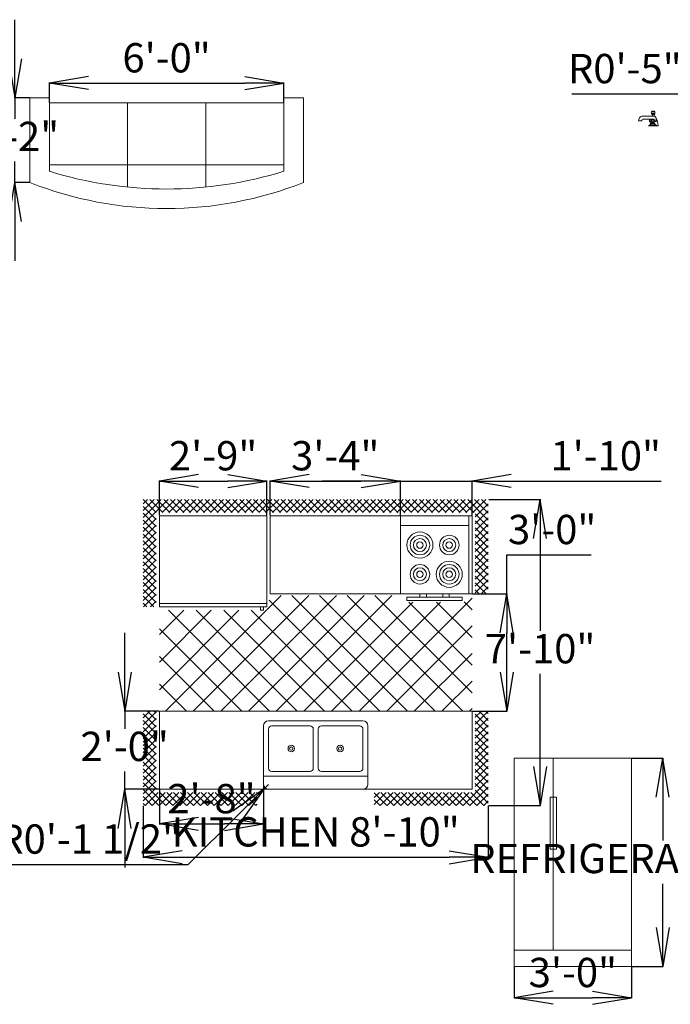
# Model space of a CAD drawing. Units: inches. Extents: x 1856 to 3350, y 1624 to 2224.
# Tile 5 of 7: x 2754 to 2954, y 1635 to 1937. Entities that reach past the tile are written whole.
import ezdxf

# ---------------------------------------------------------------- set-up
doc = ezdxf.new("R2010")
doc.units = ezdxf.units.IN
for name, color, linetype, lineweight in [('A-ANNO-DIMS', 2, 'Continuous', 18), ('A-EQPM', 3, 'Continuous', 18), ('A-FLOR-FIXT', 3, 'Continuous', 18), ('A-FURN', 3, 'Continuous', 18)]:
    doc.layers.add(name, color=color, linetype=linetype, lineweight=lineweight)
doc.styles.get("Standard").update_dxf_attribs({"font": 'arial.ttf'})
doc.dimstyles.new('ISO-25', dxfattribs={"dimtxt": 9, "dimasz": 12, "dimexe": 0.125, "dimexo": 0.125, "dimgap": 2, "dimtad": 1, "dimtih": 1, "dimtoh": 1, "dimdec": 1, "dimzin": 11, "dimlunit": 4, "dimtxsty": 'Standard', "dimblk": 'OPEN', "dimcen": -0.125, "dimadec": 0, "dimazin": 0, "dimtfac": 1, "dimtdec": 1, "dimtmove": 0, "dimatfit": 3, "dimfxl": 1, "dimarcsym": 0})

# ---------------------------------------------------------------- blocks, each defined once
blk = doc.blocks.new('Refrigerator-2 door - 36 in front')
for p, q in [((12, 5), (12, 64)), ((0, 5), (36, 5))]:
    blk.add_line(p, q)
for points in [[(0, 0), (0, 64), (36, 64), (36, 0)], [(11, 36), (11, 52), (13, 52), (13, 36)]]:
    blk.add_lwpolyline(points, close=True)
blk = doc.blocks.new('Kitchen Layout - 7 x 8 ft')
for p, q in [((-5, 81.32), (2.68, 89)), ((-5, 83.44), (0.56, 89)), ((-5, 85.56), (-1.56, 89)), ((-5, 87.68), (-3.68, 89)), ((-1, 84.97), (-5, 88.97)), ((1.09, 85), (-2.91, 89)), ((3.21, 85), (-0.79, 89)), ((0.81, 85), (4.81, 89)), ((5.34, 85), (1.34, 89)), ((2.93, 85), (6.93, 89)), ((7.46, 85), (3.46, 89)), ((5.05, 85), (9.05, 89)), ((9.58, 85), (5.58, 89)), ((7.17, 85), (11.17, 89)), ((11.7, 85), (7.7, 89)), ((9.29, 85), (13.29, 89)), ((13.82, 85), (9.82, 89)), ((11.41, 85), (15.41, 89)), ((15.94, 85), (11.94, 89)), ((13.53, 85), (17.53, 89)), ((18.06, 85), (14.06, 89)), ((15.65, 85), (19.65, 89)), ((20.18, 85), (16.18, 89)), ((17.78, 85), (21.78, 89)), ((22.31, 85), (18.31, 89)), ((19.9, 85), (23.9, 89)), ((24.43, 85), (20.43, 89)), ((22.02, 85), (26.02, 89)), ((26.55, 85), (22.55, 89)), ((24.14, 85), (28.14, 89)), ((28.67, 85), (24.67, 89)), ((26.26, 85), (30.26, 89)), ((30.79, 85), (26.79, 89)), ((28.38, 85), (32.38, 89)), ((32.91, 85), (28.91, 89)), ((30.5, 85), (34.5, 89)), ((35.03, 85), (31.03, 89)), ((32.63, 85), (36.63, 89)), ((37.16, 85), (33.16, 89)), ((34.75, 85), (38.75, 89)), ((39.28, 85), (35.28, 89)), ((36.87, 85), (40.87, 89)), ((41.4, 85), (37.4, 89)), ((38.99, 85), (42.99, 89)), ((43.52, 85), (39.52, 89)), ((41.11, 85), (45.11, 89)), ((45.64, 85), (41.64, 89)), ((43.23, 85), (47.23, 89)), ((47.76, 85), (43.76, 89)), ((45.35, 85), (49.35, 89)), ((49.88, 85), (45.88, 89)), ((47.47, 85), (51.47, 89)), ((52, 85), (48, 89)), ((49.6, 85), (53.6, 89)), ((54.13, 85), (50.13, 89)), ((51.72, 85), (55.72, 89)), ((56.25, 85), (52.25, 89)), ((53.84, 85), (57.84, 89)), ((58.37, 85), (54.37, 89)), ((55.96, 85), (59.96, 89)), ((60.49, 85), (56.49, 89)), ((58.08, 85), (62.08, 89)), ((62.61, 85), (58.61, 89)), ((60.2, 85), (64.2, 89)), ((64.73, 85), (60.73, 89)), ((62.32, 85), (66.32, 89)), ((66.85, 85), (62.85, 89)), ((64.45, 85), (68.45, 89)), ((68.97, 85), (64.97, 89)), ((66.57, 85), (70.57, 89)), ((71.1, 85), (67.1, 89)), ((68.69, 85), (72.69, 89)), ((73.22, 85), (69.22, 89)), ((70.81, 85), (74.81, 89)), ((75.34, 85), (71.34, 89)), ((72.93, 85), (76.93, 89)), ((77.46, 85), (73.46, 89)), ((75.05, 85), (79.05, 89)), ((79.58, 85), (75.58, 89)), ((77.17, 85), (81.17, 89)), ((81.7, 85), (77.7, 89)), ((79.29, 85), (83.29, 89)), ((83.82, 85), (79.82, 89)), ((81.42, 85), (85.42, 89)), ((85.95, 85), (81.95, 89)), ((83.54, 85), (87.54, 89)), ((88.07, 85), (84.07, 89)), ((85.66, 85), (89.66, 89)), ((90.19, 85), (86.19, 89)), ((87.78, 85), (91.78, 89)), ((92.31, 85), (88.31, 89)), ((89.9, 85), (93.9, 89)), ((94.43, 85), (90.43, 89)), ((92.02, 85), (96.02, 89)), ((96.55, 85), (92.55, 89)), ((94.14, 85), (98.14, 89)), ((101, 82.67), (94.67, 89)), ((96.27, 85), (100.27, 89)), ((101, 84.79), (96.79, 89)), ((101, 86.92), (98.92, 89)), ((-1, 82.85), (-5, 86.85)), ((-1, 80.73), (-5, 84.73)), ((97, 83.61), (101, 87.61)), ((97, 81.49), (101, 85.49)), ((-5, 79.19), (-1, 83.19)), ((-1, 78.61), (-5, 82.61)), ((34, 84), (96, 84)), ((34, 60), (34, 84)), ((96, 84), (96, 60)), ((101, 80.55), (97, 84.55)), ((97, 79.37), (101, 83.37)), ((101, 78.43), (97, 82.43)), ((-5, 77.07), (-1, 81.07)), ((-1, 76.49), (-5, 80.49)), ((-5, 74.95), (-1, 78.95)), ((74, 81), (95, 81)), ((97, 77.25), (101, 81.25)), ((101, 76.31), (97, 80.31)), ((97, 75.13), (101, 79.13)), ((-1, 74.36), (-5, 78.36)), ((-5, 72.83), (-1, 76.83)), ((-1, 72.24), (-5, 76.24)), ((101, 74.19), (97, 78.19)), ((97, 73.01), (101, 77.01)), ((101, 72.07), (97, 76.07)), ((-5, 70.71), (-1, 74.71)), ((-1, 70.12), (-5, 74.12)), ((-5, 68.59), (-1, 72.59)), ((97, 70.89), (101, 74.89)), ((101, 69.95), (97, 73.95)), ((97, 68.76), (101, 72.76)), ((-1, 68), (-5, 72)), ((-5, 66.47), (-1, 70.47)), ((-1, 65.88), (-5, 69.88)), ((101, 67.82), (97, 71.82)), ((97, 66.64), (101, 70.64)), ((101, 65.7), (97, 69.7)), ((-5, 64.35), (-1, 68.35)), ((-1, 63.76), (-5, 67.76)), ((97, 64.52), (101, 68.52)), ((101, 63.58), (97, 67.58)), ((-5, 62.22), (-1, 66.22)), ((-1, 61.64), (-5, 65.64)), ((-5, 60.1), (-1, 64.1)), ((-1, 59.52), (-5, 63.52)), ((97, 62.4), (101, 66.4)), ((101, 61.46), (97, 65.46)), ((97, 60.28), (101, 64.28)), ((-5, 57.98), (-1, 61.98)), ((-1, 57.39), (-5, 61.39)), ((100.34, 60), (97, 63.34)), ((98.22, 60), (97, 61.22)), ((98.84, 60), (101, 62.16)), ((-1.73, 56), (-5, 59.27)), ((-4.86, 56), (-1, 59.86)), ((-2.74, 56), (-1, 57.74)), ((10.4, 24), (45.9, 59.5)), ((18.88, 24), (54.38, 59.5)), ((27.37, 24), (62.87, 59.5)), ((33.03, 55.11), (37.41, 59.5)), ((67.71, 24), (33.68, 58.04)), ((96, 60), (34, 60)), ((35.85, 24), (71.35, 59.5)), ((76.2, 24), (40.7, 59.5)), ((44.34, 24), (77.84, 57.5)), ((84.68, 24), (49.18, 59.5)), ((52.82, 24), (86.32, 57.5)), ((93.17, 24), (57.67, 59.5)), ((61.31, 24), (96, 58.69)), ((96, 29.65), (66.15, 59.5)), ((96, 38.14), (76.64, 57.5)), ((80, 60), (80, 59)), ((82, 59), (82, 60)), ((96, 46.63), (85.13, 57.5)), ((87, 59), (87, 60)), ((89, 60), (89, 59)), ((96, 55.11), (93.57, 57.54)), ((100.96, 60), (101, 60.04)), ((-3.85, 56), (-5, 57.15)), ((0, 57), (33, 57)), ((0, 30.57), (24.43, 55)), ((0, 39.06), (15.94, 55)), ((0, 47.54), (7.46, 55)), ((1.91, 24), (32.91, 55)), ((33.77, 24), (2.77, 55)), ((42.26, 24), (11.26, 55)), ((50.74, 24), (19.74, 55)), ((59.23, 24), (28.23, 55)), ((31, 55), (31, 56)), ((32, 55), (31, 55)), ((32, 56), (32, 55)), ((25.29, 24), (0, 49.29)), ((69.79, 24), (96, 50.21)), ((16.8, 24), (0, 40.8)), ((78.28, 24), (96, 41.72)), ((8.32, 24), (0, 32.32)), ((86.76, 24), (96, 33.24)), ((95.25, 24), (96, 24.75)), ((-5, 21.92), (-2.92, 24)), ((-5, 19.8), (-1, 23.8)), ((-1, 19.21), (-5, 23.21)), ((-5, 17.68), (-1, 21.68)), ((-1, 21.33), (-3.67, 24)), ((-1, 23.45), (-1.55, 24)), ((0, 24), (96, 24)), ((0, 0), (0, 24)), ((96, 24), (96, 0)), ((97, 22.1), (98.9, 24)), ((97, 19.97), (101, 23.97)), ((101, 19.03), (97, 23.03)), ((97, 17.85), (101, 21.85)), ((101, 21.16), (98.16, 24)), ((101, 23.28), (100.28, 24)), ((-1, 17.09), (-5, 21.09)), ((-5, 15.55), (-1, 19.55)), ((-1, 14.97), (-5, 18.97)), ((47.25, 6.5), (47.25, 18.5)), ((48.75, 18.5), (48.75, 6.5)), ((101, 16.91), (97, 20.91)), ((97, 15.73), (101, 19.73)), ((101, 14.79), (97, 18.79)), ((-5, 13.43), (-1, 17.43)), ((-1, 12.85), (-5, 16.85)), ((-5, 11.31), (-1, 15.31)), ((97, 13.61), (101, 17.61)), ((101, 12.67), (97, 16.67)), ((97, 11.49), (101, 15.49)), ((-1, 10.73), (-5, 14.73)), ((-5, 9.19), (-1, 13.19)), ((-1, 8.6), (-5, 12.6)), ((101, 10.55), (97, 14.55)), ((97, 9.37), (101, 13.37)), ((101, 8.43), (97, 12.43)), ((-5, 7.07), (-1, 11.07)), ((-1, 6.48), (-5, 10.48)), ((97, 7.25), (101, 11.25)), ((101, 6.31), (97, 10.31)), ((97, 5.12), (101, 9.12)), ((-5, 4.95), (-1, 8.95)), ((-1, 4.36), (-5, 8.36)), ((-5, 2.83), (-1, 6.83)), ((-1, 2.24), (-5, 6.24)), ((101, 4.18), (97, 8.18)), ((97, 3), (101, 7)), ((101, 2.06), (97, 6.06)), ((-5, 0.71), (-1, 4.71)), ((-1, 0.12), (-5, 4.12)), ((64, 4), (32, 4)), ((97, 0.88), (101, 4.88)), ((101, -0.06), (97, 3.94)), ((-5, -1.42), (-1, 2.58)), ((2, -5), (-5, 2)), ((-5, -3.54), (-1, 0.46)), ((96, 0), (0, 0)), ((93.24, -5), (101, 2.76)), ((95.36, -5), (101, 0.64)), ((101, -2.18), (97, 1.82)), ((-0.12, -5), (-5, -0.12)), ((-2.25, -5), (-5, -2.25)), ((-4.34, -5), (-0.34, -1)), ((-2.22, -5), (1.78, -1)), ((-0.1, -5), (3.9, -1)), ((4.12, -5), (0.12, -1)), ((2.02, -5), (6.02, -1)), ((6.24, -5), (2.24, -1)), ((4.14, -5), (8.14, -1)), ((8.36, -5), (4.36, -1)), ((6.27, -5), (10.27, -1)), ((10.48, -5), (6.48, -1)), ((8.39, -5), (12.39, -1)), ((12.6, -5), (8.6, -1)), ((10.51, -5), (14.51, -1)), ((14.73, -5), (10.73, -1)), ((12.63, -5), (16.63, -1)), ((16.85, -5), (12.85, -1)), ((14.75, -5), (18.75, -1)), ((18.97, -5), (14.97, -1)), ((16.87, -5), (20.87, -1)), ((21.09, -5), (17.09, -1)), ((18.99, -5), (22.99, -1)), ((23.21, -5), (19.21, -1)), ((21.11, -5), (25.11, -1)), ((25.33, -5), (21.33, -1)), ((23.24, -5), (27.24, -1)), ((27.45, -5), (23.45, -1)), ((25.36, -5), (29.36, -1)), ((29.57, -5), (25.57, -1)), ((27.48, -5), (30, -2.48)), ((30, -3.3), (27.7, -1)), ((30, -1.18), (29.82, -1)), ((66, -2.54), (67.54, -1)), ((66, -4.66), (69.66, -1)), ((69.88, -5), (66, -1.12)), ((67.78, -5), (71.78, -1)), ((72, -5), (68, -1)), ((69.9, -5), (73.9, -1)), ((74.12, -5), (70.12, -1)), ((72.03, -5), (76.03, -1)), ((76.24, -5), (72.24, -1)), ((74.15, -5), (78.15, -1)), ((78.36, -5), (74.36, -1)), ((76.27, -5), (80.27, -1)), ((80.49, -5), (76.49, -1)), ((78.39, -5), (82.39, -1)), ((82.61, -5), (78.61, -1)), ((80.51, -5), (84.51, -1)), ((84.73, -5), (80.73, -1)), ((82.63, -5), (86.63, -1)), ((86.85, -5), (82.85, -1)), ((84.75, -5), (88.75, -1)), ((88.97, -5), (84.97, -1)), ((86.88, -5), (90.88, -1)), ((91.09, -5), (87.09, -1)), ((89, -5), (93, -1)), ((93.21, -5), (89.21, -1)), ((91.12, -5), (95.12, -1)), ((95.34, -5), (91.34, -1)), ((97.46, -5), (93.46, -1)), ((99.58, -5), (95.58, -1)), ((101, -4.3), (97, -0.3)), ((97.48, -5), (101, -1.48)), ((-4.37, -5), (-5, -4.37)), ((29.6, -5), (30, -4.6)), ((67.76, -5), (66, -3.24)), ((99.6, -5), (101, -3.6))]:
    blk.add_line(p, q)
for points in [[(0, 56), (0, 84), (33, 84), (33, 56)], [(74, 60), (74, 84), (95, 84), (95, 60)], [(76, 58), (76, 59), (93, 59), (93, 58)]]:
    blk.add_lwpolyline(points, close=True)
for points in [[(32, 1.5), (32, 19.5)], [(33.5, 21), (62.5, 21)], [(33.5, 6.5), (33.5, 18.5)], [(34.5, 19.5), (46.25, 19.5)], [(49.75, 19.5), (61.5, 19.5)], [(62.5, 18.5), (62.5, 6.5)], [(64, 19.5), (64, 1.5)], [(46.25, 5.5), (34.5, 5.5)], [(61.5, 5.5), (49.75, 5.5)], [(62.5, 0), (33.5, 0)]]:
    blk.add_lwpolyline(points)
for centre, radius in [((80, 75), 4), ((80, 75), 3), ((80, 75), 2), ((80, 75), 1), ((89, 75), 3), ((89, 75), 2), ((89, 75), 1), ((89, 66), 4), ((80, 66), 3), ((80, 66), 2), ((80, 66), 1), ((89, 66), 3), ((89, 66), 2), ((89, 66), 1), ((40.5, 12.5), 1), ((40.5, 12.5), 0.5), ((55.5, 12.5), 1), ((55.5, 12.5), 0.5)]:
    blk.add_circle(centre, radius)
for centre, radius, start, end in [((33.5, 19.5), 1.5, 90, 180), ((34.5, 18.5), 1, 90, 180), ((46.25, 18.5), 1, 0, 90), ((49.75, 18.5), 1, 90, 180), ((61.5, 18.5), 1, 0, 90), ((62.5, 19.5), 1.5, 0, 90), ((34.5, 6.5), 1, 180, 270), ((46.25, 6.5), 1, 270, 0), ((49.75, 6.5), 1, 180, 270), ((61.5, 6.5), 1, 270, 0), ((33.5, 1.5), 1.5, 180, 270), ((62.5, 1.5), 1.5, 270, 0)]:
    blk.add_arc(centre, radius, start, end)
blk = doc.blocks.new('Sofa - Roundback 7 ft.')
for p, q in [((-12.00002, -32.4421), (-12.00003, -6.5971)), ((11.99997, -32.4421), (11.99998, -6.5971)), ((-36.000027, -34), (-36.000027, -11.4696)), ((35.99998, -34), (35.99998, -11.4696)), ((-35.999844, -13.3819), (35.9998, -13.3819)), ((-36.000027, -32.4421), (35.99998, -32.4421))]:
    blk.add_line(p, q)
for points in [[(-36.000027, -34), (-42.000027, -34), (-42.000027, -8)], [(41.99998, -8), (41.99998, -34), (35.99998, -34)]]:
    blk.add_lwpolyline(points)
for centre, radius, start, end in [((0, -114.25), 114.25, 68.43141, 111.5686), ((-0.00001, -127.1968), 121.1968, 72.72033, 107.2797)]:
    blk.add_arc(centre, radius, start, end)
blk = doc.blocks.new('Faucet - Bathroom side')
for p, q in [((-0.625, 4.25), (0.375, 4.25)), ((0.375, 3.75), (-0.625, 3.75)), ((-0.375, 3), (-0.375, 3.5)), ((0.125, 3.5), (0.125, 3)), ((-1.625, 0), (-1.375, 0)), ((-1.375, 0), (1.375, 0)), ((-0.88366, 0.25), (0.88424, 0.25)), ((-0.625, 3), (3.375, 3)), ((-0.375, 1.625), (-0.625, 1.625)), ((-0.375, 1.375), (-0.625, 1.375)), ((0.48078, 0.75), (-0.47286, 0.75)), ((2.875, 2), (0.375, 2)), ((0.375, 1.625), (0.625, 1.625)), ((0.375, 1.375), (0.625, 1.375)), ((4.375, 1.5), (3.375, 1.5))]:
    blk.add_line(p, q)
for points in [[(-0.625, 3.75), (-0.625, 4.25)], [(-0.375, 4.5), (0.125, 4.5)], [(0.125, 3.5), (-0.375, 3.5)], [(0.375, 4.25), (0.375, 3.75)]]:
    blk.add_lwpolyline(points)
blk.add_lwpolyline([(-0.375, 1), (-0.375, 2), (0.375, 2), (0.375, 1)], close=True)
for centre in [(-0.875, 1.5), (0, 1.5), (0.875, 1.5)]:
    blk.add_circle(centre, 0.27951)
for centre, radius, start, end in [((-0.38253, 4.2575), 0.24259, 88.22243, 181.7776), ((-0.38253, 3.7424), 0.24259, 178.2224, 271.7776), ((0.13252, 4.2575), 0.24259, 358.2224, 91.77757), ((0.13252, 3.7424), 0.24259, 268.2224, 1.777565), ((3.45929, -0.0281), 5.08436, 143.4467, 179.6834), ((-1.75, 1.375), 1.42522, 285.2551, 344.7449), ((1.75, 1.375), 1.42522, 195.2551, 254.7449), ((-2.49562, -0.286), 3.38273, 9.709485, 29.48735), ((2.96867, 1.5936), 0.41699, 347.0192, 102.9808), ((2.70708, 1.4714), 1.66816, 0.9827695, 66.39737)]:
    blk.add_arc(centre, radius, start, end)
blk = doc.blocks.new('_Open')
at = {"color": 0, "linetype": 'ByBlock', "lineweight": -2}
for p, q in [((-1, 0.167), (0, 0)), ((-1, -0.167), (0, 0)), ((0, 0), (-1, 0))]:
    blk.add_line(p, q, dxfattribs=at)
blk = doc.blocks.new('*D46')
at = {"layer": 'A-ANNO-DIMS', "color": 0, "lineweight": -2, "transparency": 16777216}
for p, q in [((2942.46, 1710.58), (2952.06, 1710.58)), ((2951.94, 1698.58), (2951.94, 1685.23)), ((2951.94, 1658.58), (2951.94, 1671.92)), ((2942.46, 1646.58), (2952.06, 1646.58))]:
    blk.add_line(p, q, dxfattribs=at)
at = {"layer": 'Defpoints', "color": 0, "transparency": 16777216}
for p in [(2942.34, 1710.58), (2951.94, 1710.58), (2942.34, 1646.58)]:
    blk.add_point(p, dxfattribs=at)
at = {"layer": 'A-ANNO-DIMS', "color": 0, "lineweight": -2, "transparency": 16777216, "xscale": 12, "yscale": 12, "zscale": 12}
for p, rotation in [((2951.94, 1710.58), 90), ((2951.94, 1646.58), 270)]:
    blk.add_blockref('_Open', p, dxfattribs=dict(at, rotation=rotation))
at = {"layer": 'A-ANNO-DIMS', "color": 0, "transparency": 16777216, "insert": (2951.94, 1678.58), "char_height": 9, "attachment_point": 5}
blk.add_mtext('REFRIGERATOR 5\'-4"', dxfattribs=at)
blk = doc.blocks.new('*D47')
at = {"layer": 'A-ANNO-DIMS', "color": 0, "lineweight": -2, "transparency": 16777216}
for p, q in [((2906.34, 1646.45), (2906.34, 1636.85)), ((2942.34, 1646.45), (2942.34, 1636.85)), ((2918.34, 1636.98), (2930.34, 1636.98))]:
    blk.add_line(p, q, dxfattribs=at)
at = {"layer": 'Defpoints', "color": 0, "transparency": 16777216}
for p in [(2906.34, 1646.58), (2942.34, 1646.58), (2942.34, 1636.98)]:
    blk.add_point(p, dxfattribs=at)
at = {"layer": 'A-ANNO-DIMS', "color": 0, "lineweight": -2, "transparency": 16777216, "xscale": 12, "yscale": 12, "zscale": 12, "rotation": 180}
blk.add_blockref('_Open', (2906.34, 1636.98), dxfattribs=at)
at = {"layer": 'A-ANNO-DIMS', "color": 0, "lineweight": -2, "transparency": 16777216, "xscale": 12, "yscale": 12, "zscale": 12}
blk.add_blockref('_Open', (2942.34, 1636.98), dxfattribs=at)
at = {"layer": 'A-ANNO-DIMS', "color": 0, "transparency": 16777216, "insert": (2924.34, 1643.58), "char_height": 9, "attachment_point": 5}
blk.add_mtext('3\'-0"', dxfattribs=at)
blk = doc.blocks.new('*D48')
at = {"layer": 'A-ANNO-DIMS', "color": 0, "lineweight": -2, "transparency": 16777216}
for p, q in [((2792.38, 1695.89), (2792.38, 1679.99)), ((2898.38, 1695.89), (2898.38, 1679.99)), ((2804.38, 1680.11), (2886.38, 1680.11))]:
    blk.add_line(p, q, dxfattribs=at)
at = {"layer": 'Defpoints', "color": 0, "transparency": 16777216}
for p in [(2792.38, 1696.01), (2898.38, 1696.01), (2898.38, 1680.11)]:
    blk.add_point(p, dxfattribs=at)
at = {"layer": 'A-ANNO-DIMS', "color": 0, "lineweight": -2, "transparency": 16777216, "xscale": 12, "yscale": 12, "zscale": 12, "rotation": 180}
blk.add_blockref('_Open', (2792.38, 1680.11), dxfattribs=at)
at = {"layer": 'A-ANNO-DIMS', "color": 0, "lineweight": -2, "transparency": 16777216, "xscale": 12, "yscale": 12, "zscale": 12}
blk.add_blockref('_Open', (2898.38, 1680.11), dxfattribs=at)
at = {"layer": 'A-ANNO-DIMS', "color": 0, "transparency": 16777216, "insert": (2845.38, 1686.76), "char_height": 9, "attachment_point": 5}
blk.add_mtext('KITCHEN 8\'-10"', dxfattribs=at)
blk = doc.blocks.new('*D49')
at = {"layer": 'A-ANNO-DIMS', "color": 0, "lineweight": -2, "transparency": 16777216}
for p, q in [((2898.51, 1790.01), (2914.41, 1790.01)), ((2914.28, 1778.01), (2914.28, 1749.61)), ((2914.28, 1708.01), (2914.28, 1736.42)), ((2898.51, 1696.01), (2914.41, 1696.01))]:
    blk.add_line(p, q, dxfattribs=at)
at = {"layer": 'Defpoints', "color": 0, "transparency": 16777216}
for p in [(2898.38, 1790.01), (2914.28, 1790.01), (2898.38, 1696.01)]:
    blk.add_point(p, dxfattribs=at)
at = {"layer": 'A-ANNO-DIMS', "color": 0, "lineweight": -2, "transparency": 16777216, "xscale": 12, "yscale": 12, "zscale": 12}
for p, rotation in [((2914.28, 1790.01), 90), ((2914.28, 1696.01), 270)]:
    blk.add_blockref('_Open', p, dxfattribs=dict(at, rotation=rotation))
at = {"layer": 'A-ANNO-DIMS', "color": 0, "transparency": 16777216, "insert": (2914.28, 1743.01), "char_height": 9, "attachment_point": 5}
blk.add_mtext('7\'-10"', dxfattribs=at)
blk = doc.blocks.new('*D75')
at = {"layer": 'A-ANNO-DIMS', "color": 0, "lineweight": -2, "transparency": 16777216}
for p, q in [((2763.6, 1911.88), (2763.6, 1917.99)), ((2775.6, 1917.87), (2823.6, 1917.87)), ((2835.6, 1911.88), (2835.6, 1917.99))]:
    blk.add_line(p, q, dxfattribs=at)
at = {"layer": 'Defpoints', "color": 0, "transparency": 16777216}
for p in [(2835.6, 1917.87), (2763.6, 1911.76), (2835.6, 1911.76)]:
    blk.add_point(p, dxfattribs=at)
at = {"layer": 'A-ANNO-DIMS', "color": 0, "lineweight": -2, "transparency": 16777216, "xscale": 12, "yscale": 12, "zscale": 12, "rotation": 180}
blk.add_blockref('_Open', (2763.6, 1917.87), dxfattribs=at)
at = {"layer": 'A-ANNO-DIMS', "color": 0, "lineweight": -2, "transparency": 16777216, "xscale": 12, "yscale": 12, "zscale": 12}
blk.add_blockref('_Open', (2835.6, 1917.87), dxfattribs=at)
at = {"layer": 'A-ANNO-DIMS', "color": 0, "transparency": 16777216, "insert": (2799.6, 1924.46), "char_height": 9, "attachment_point": 5}
blk.add_mtext('6\'-0"', dxfattribs=at)
blk = doc.blocks.new('*D76')
at = {"layer": 'A-ANNO-DIMS', "color": 0, "lineweight": -2, "transparency": 16777216}
for p, q in [((2753.05, 1925.32), (2753.05, 1937.32)), ((2757.48, 1913.32), (2752.93, 1913.32)), ((2753.05, 1913.32), (2753.05, 1906.83)), ((2753.05, 1887.32), (2753.05, 1893.8)), ((2757.48, 1887.32), (2752.93, 1887.32)), ((2753.05, 1875.32), (2753.05, 1863.32))]:
    blk.add_line(p, q, dxfattribs=at)
at = {"layer": 'Defpoints', "color": 0, "transparency": 16777216}
for p in [(2757.6, 1913.32), (2753.05, 1887.32), (2757.6, 1887.32)]:
    blk.add_point(p, dxfattribs=at)
at = {"layer": 'A-ANNO-DIMS', "color": 0, "lineweight": -2, "transparency": 16777216, "xscale": 12, "yscale": 12, "zscale": 12}
for p, rotation in [((2753.05, 1913.32), 270), ((2753.05, 1887.32), 90)]:
    blk.add_blockref('_Open', p, dxfattribs=dict(at, rotation=rotation))
at = {"layer": 'A-ANNO-DIMS', "color": 0, "transparency": 16777216, "insert": (2753.05, 1900.32), "char_height": 9, "attachment_point": 5}
blk.add_mtext('2\'-2"', dxfattribs=at)
blk = doc.blocks.new('*D81')
at = {"layer": 'A-ANNO-DIMS', "color": 0, "lineweight": -2, "transparency": 16777216}
for p, q in [((2786.73, 1737.01), (2786.73, 1749.01)), ((2797.26, 1725.01), (2786.61, 1725.01)), ((2786.73, 1725.01), (2786.73, 1719.61)), ((2786.73, 1701.01), (2786.73, 1706.42)), ((2797.26, 1701.01), (2786.61, 1701.01)), ((2786.73, 1689.01), (2786.73, 1677.01))]:
    blk.add_line(p, q, dxfattribs=at)
at = {"layer": 'Defpoints', "color": 0, "transparency": 16777216}
for p in [(2786.73, 1725.01), (2797.38, 1725.01), (2797.38, 1701.01)]:
    blk.add_point(p, dxfattribs=at)
at = {"layer": 'A-ANNO-DIMS', "color": 0, "lineweight": -2, "transparency": 16777216, "xscale": 12, "yscale": 12, "zscale": 12}
for p, rotation in [((2786.73, 1725.01), 270), ((2786.73, 1701.01), 90)]:
    blk.add_blockref('_Open', p, dxfattribs=dict(at, rotation=rotation))
at = {"layer": 'A-ANNO-DIMS', "color": 0, "transparency": 16777216, "insert": (2786.73, 1713.01), "char_height": 9, "attachment_point": 5}
blk.add_mtext('2\'-0"', dxfattribs=at)
blk = doc.blocks.new('*D82')
at = {"layer": 'A-ANNO-DIMS', "color": 0, "lineweight": -2, "transparency": 16777216}
for p, q in [((2904.03, 1761.01), (2904.03, 1773.01)), ((2904.03, 1773.01), (2929.95, 1773.01)), ((2893.51, 1761.01), (2904.16, 1761.01)), ((2904.03, 1737.01), (2904.03, 1749.01)), ((2893.51, 1725.01), (2904.16, 1725.01))]:
    blk.add_line(p, q, dxfattribs=at)
at = {"layer": 'Defpoints', "color": 0, "transparency": 16777216}
for p in [(2893.38, 1761.01), (2904.03, 1761.01), (2893.38, 1725.01)]:
    blk.add_point(p, dxfattribs=at)
at = {"layer": 'A-ANNO-DIMS', "color": 0, "lineweight": -2, "transparency": 16777216, "xscale": 12, "yscale": 12, "zscale": 12}
for p, rotation in [((2904.03, 1761.01), 90), ((2904.03, 1725.01), 270)]:
    blk.add_blockref('_Open', p, dxfattribs=dict(at, rotation=rotation))
at = {"layer": 'A-ANNO-DIMS', "color": 0, "transparency": 16777216, "insert": (2917.99, 1779.61), "char_height": 9, "attachment_point": 5}
blk.add_mtext('3\'-0"', dxfattribs=at)
blk = doc.blocks.new('*D83')
at = {"layer": 'A-ANNO-DIMS', "color": 0, "lineweight": -2, "transparency": 16777216}
for p, q in [((2797.38, 1785.14), (2797.38, 1795.79)), ((2809.38, 1795.66), (2818.38, 1795.66)), ((2830.38, 1785.14), (2830.38, 1795.79))]:
    blk.add_line(p, q, dxfattribs=at)
at = {"layer": 'Defpoints', "color": 0, "transparency": 16777216}
for p in [(2830.38, 1795.66), (2797.38, 1785.01), (2830.38, 1785.01)]:
    blk.add_point(p, dxfattribs=at)
at = {"layer": 'A-ANNO-DIMS', "color": 0, "lineweight": -2, "transparency": 16777216, "xscale": 12, "yscale": 12, "zscale": 12, "rotation": 180}
blk.add_blockref('_Open', (2797.38, 1795.66), dxfattribs=at)
at = {"layer": 'A-ANNO-DIMS', "color": 0, "lineweight": -2, "transparency": 16777216, "xscale": 12, "yscale": 12, "zscale": 12}
blk.add_blockref('_Open', (2830.38, 1795.66), dxfattribs=at)
at = {"layer": 'A-ANNO-DIMS', "color": 0, "transparency": 16777216, "insert": (2813.88, 1802.26), "char_height": 9, "attachment_point": 5}
blk.add_mtext('2\'-9"', dxfattribs=at)
blk = doc.blocks.new('*D84')
at = {"layer": 'A-ANNO-DIMS', "color": 0, "lineweight": -2, "transparency": 16777216}
for p, q in [((2831.38, 1785.14), (2831.38, 1795.79)), ((2843.38, 1795.66), (2859.38, 1795.66)), ((2871.38, 1785.14), (2871.38, 1795.79))]:
    blk.add_line(p, q, dxfattribs=at)
at = {"layer": 'Defpoints', "color": 0, "transparency": 16777216}
for p in [(2871.38, 1795.66), (2831.38, 1785.01), (2871.38, 1785.01)]:
    blk.add_point(p, dxfattribs=at)
at = {"layer": 'A-ANNO-DIMS', "color": 0, "lineweight": -2, "transparency": 16777216, "xscale": 12, "yscale": 12, "zscale": 12, "rotation": 180}
blk.add_blockref('_Open', (2831.38, 1795.66), dxfattribs=at)
at = {"layer": 'A-ANNO-DIMS', "color": 0, "lineweight": -2, "transparency": 16777216, "xscale": 12, "yscale": 12, "zscale": 12}
blk.add_blockref('_Open', (2871.38, 1795.66), dxfattribs=at)
at = {"layer": 'A-ANNO-DIMS', "color": 0, "transparency": 16777216, "insert": (2851.38, 1802.26), "char_height": 9, "attachment_point": 5}
blk.add_mtext('3\'-4"', dxfattribs=at)
blk = doc.blocks.new('*D85')
at = {"layer": 'A-ANNO-DIMS', "color": 0, "lineweight": -2, "transparency": 16777216}
for p, q in [((2859.38, 1795.66), (2847.38, 1795.66)), ((2871.38, 1785.14), (2871.38, 1795.79)), ((2871.38, 1795.66), (2893.38, 1795.66)), ((2893.38, 1785.14), (2893.38, 1795.79)), ((2905.38, 1795.66), (2951.45, 1795.66))]:
    blk.add_line(p, q, dxfattribs=at)
at = {"layer": 'Defpoints', "color": 0, "transparency": 16777216}
for p in [(2893.38, 1795.66), (2871.38, 1785.01), (2893.38, 1785.01)]:
    blk.add_point(p, dxfattribs=at)
at = {"layer": 'A-ANNO-DIMS', "color": 0, "lineweight": -2, "transparency": 16777216, "xscale": 12, "yscale": 12, "zscale": 12}
blk.add_blockref('_Open', (2871.38, 1795.66), dxfattribs=at)
at = {"layer": 'A-ANNO-DIMS', "color": 0, "lineweight": -2, "transparency": 16777216, "xscale": 12, "yscale": 12, "zscale": 12, "rotation": 180}
blk.add_blockref('_Open', (2893.38, 1795.66), dxfattribs=at)
at = {"layer": 'A-ANNO-DIMS', "color": 0, "transparency": 16777216, "insert": (2934.42, 1802.26), "char_height": 9, "attachment_point": 5}
blk.add_mtext('1\'-10"', dxfattribs=at)
blk = doc.blocks.new('*D86')
at = {"layer": 'A-ANNO-DIMS', "color": 0, "lineweight": -2, "transparency": 16777216}
for p, q in [((2829.38, 1702.39), (2829.38, 1690.24)), ((2797.38, 1700.89), (2797.38, 1690.24)), ((2809.38, 1690.36), (2817.38, 1690.36))]:
    blk.add_line(p, q, dxfattribs=at)
at = {"layer": 'Defpoints', "color": 0, "transparency": 16777216}
for p in [(2829.38, 1702.51), (2797.38, 1701.01), (2829.38, 1690.36)]:
    blk.add_point(p, dxfattribs=at)
at = {"layer": 'A-ANNO-DIMS', "color": 0, "lineweight": -2, "transparency": 16777216, "xscale": 12, "yscale": 12, "zscale": 12, "rotation": 180}
blk.add_blockref('_Open', (2797.38, 1690.36), dxfattribs=at)
at = {"layer": 'A-ANNO-DIMS', "color": 0, "lineweight": -2, "transparency": 16777216, "xscale": 12, "yscale": 12, "zscale": 12}
blk.add_blockref('_Open', (2829.38, 1690.36), dxfattribs=at)
at = {"layer": 'A-ANNO-DIMS', "color": 0, "transparency": 16777216, "insert": (2813.38, 1696.96), "char_height": 9, "attachment_point": 5}
blk.add_mtext('2\'-8"', dxfattribs=at)
blk = doc.blocks.new('*D101')
at = {"layer": 'A-ANNO-DIMS', "color": 0, "lineweight": -2, "transparency": 16777216}
for p, q in [((2830.88, 1702.51), (2829.82, 1701.45)), ((2806.26, 1677.9), (2821.33, 1692.97)), ((2731.06, 1677.9), (2806.26, 1677.9))]:
    blk.add_line(p, q, dxfattribs=at)
at = {"layer": 'Defpoints', "color": 0, "transparency": 16777216}
for p in [(2830.88, 1702.51), (2829.82, 1701.45)]:
    blk.add_point(p, dxfattribs=at)
at = {"layer": 'A-ANNO-DIMS', "color": 0, "lineweight": -2, "transparency": 16777216, "xscale": 12, "yscale": 12, "zscale": 12, "rotation": 44.99157303797349}
blk.add_blockref('_Open', (2829.82, 1701.45), dxfattribs=at)
at = {"layer": 'A-ANNO-DIMS', "color": 0, "transparency": 16777216, "insert": (2767.66, 1684.56), "char_height": 9, "attachment_point": 5}
blk.add_mtext('4X R0\'-1 1/2"', dxfattribs=at)
blk = doc.blocks.new('*D109')
at = {"layer": 'A-ANNO-DIMS', "color": 0, "lineweight": -2, "transparency": 16777216}
for p, q in [((2924.02, 1914.54), (2958.56, 1914.54)), ((2958.56, 1914.54), (2969.94, 1910.75)), ((2986.15, 1905.34), (2981.32, 1906.95))]:
    blk.add_line(p, q, dxfattribs=at)
at = {"layer": 'Defpoints', "color": 0, "transparency": 16777216}
for p in [(2981.32, 1906.95), (2986.15, 1905.34)]:
    blk.add_point(p, dxfattribs=at)
at = {"layer": 'A-ANNO-DIMS', "color": 0, "lineweight": -2, "transparency": 16777216, "xscale": 12, "yscale": 12, "zscale": 12, "rotation": 341.5598341012926}
blk.add_blockref('_Open', (2981.32, 1906.95), dxfattribs=at)
at = {"layer": 'A-ANNO-DIMS', "color": 0, "transparency": 16777216, "insert": (2940.29, 1921.14), "char_height": 9, "attachment_point": 5}
blk.add_mtext('R0\'-5"', dxfattribs=at)

msp = doc.modelspace()

# ---------------------------------------------------------------- block references
at = {"layer": 'A-EQPM'}
msp.add_blockref('Refrigerator-2 door - 36 in front', (2906.34, 1646.58), dxfattribs=at)
at = {"layer": 'A-FLOR-FIXT', "xscale": -1}
msp.add_blockref('Faucet - Bathroom side', (2948.89, 1904.74), dxfattribs=at)
at = {"layer": 'A-FLOR-FIXT'}
msp.add_blockref('Kitchen Layout - 7 x 8 ft', (2797.38, 1701.01), dxfattribs=at)
at = {"layer": 'A-FURN', "rotation": 180}
msp.add_blockref('Sofa - Roundback 7 ft.', (2799.6, 1879.32), dxfattribs=at)

# ---------------------------------------------------------------- dimensions: what is measured, and where the dimension line sits
at = {"layer": 'A-ANNO-DIMS'}
for base, p1, p2, picture, middle in [((2753.05, 1887.32), (2757.6, 1913.32), (2757.6, 1887.32), '*D76', (2753.05, 1900.32)), ((2914.28, 1790.01), (2898.38, 1696.01), (2898.38, 1790.01), '*D49', (2914.28, 1743.01)), ((2904.03, 1761.01), (2893.38, 1725.01), (2893.38, 1761.01), '*D82', (2917.99, 1779.61)), ((2786.73, 1725.01), (2797.38, 1701.01), (2797.38, 1725.01), '*D81', (2786.73, 1713.01))]:
    dim = msp.add_linear_dim(base=base, p1=p1, p2=p2, angle=90, dimstyle='ISO-25', override={"dimdec": 1, "dimlfac": 1, "dimrnd": 0, "dimzin": 1, "dimdsep": 46, "dimlunit": 4, "dimfrac": 2}, dxfattribs=at)
    dim.commit()
    dim.dimension.update_dxf_attribs({"geometry": picture, "text_midpoint": middle})
for base, p1, p2, picture, middle in [((2835.6, 1917.87), (2763.6, 1911.76), (2835.6, 1911.76), '*D75', (2799.6, 1924.46)), ((2830.38, 1795.66), (2797.38, 1785.01), (2830.38, 1785.01), '*D83', (2813.88, 1802.26)), ((2871.38, 1795.66), (2831.38, 1785.01), (2871.38, 1785.01), '*D84', (2851.38, 1802.26)), ((2893.38, 1795.66), (2871.38, 1785.01), (2893.38, 1785.01), '*D85', (2934.42, 1802.26)), ((2829.38, 1690.36), (2797.38, 1701.01), (2829.38, 1702.51), '*D86', (2813.38, 1696.96)), ((2942.34, 1636.98), (2906.34, 1646.58), (2942.34, 1646.58), '*D47', (2924.34, 1643.58))]:
    dim = msp.add_linear_dim(base=base, p1=p1, p2=p2, dimstyle='ISO-25', override={"dimdec": 1, "dimlfac": 1, "dimrnd": 0, "dimzin": 1, "dimdsep": 46, "dimlunit": 4, "dimfrac": 2}, dxfattribs=at)
    dim.commit()
    dim.dimension.update_dxf_attribs({"geometry": picture, "text_midpoint": middle})
dim = msp.add_radius_dim(center=(2986.15, 1905.34), mpoint=(2981.32, 1906.95), dimstyle='ISO-25', override={"dimdec": 1, "dimlfac": 1, "dimrnd": 0, "dimzin": 1, "dimdsep": 46, "dimlunit": 4, "dimfrac": 2}, dxfattribs=at)
dim.commit()
dim.dimension.update_dxf_attribs({"geometry": '*D109', "text_midpoint": (2940.29, 1921.14)})
dim = msp.add_linear_dim(base=(2951.94, 1710.58), p1=(2942.34, 1646.58), p2=(2942.34, 1710.58), angle=90, text='REFRIGERATOR <>', dimstyle='ISO-25', override={"dimdec": 1, "dimlfac": 1, "dimrnd": 0, "dimzin": 1, "dimdsep": 46, "dimlunit": 4, "dimfrac": 2}, dxfattribs=at)
dim.commit()
dim.dimension.update_dxf_attribs({"geometry": '*D46', "text_midpoint": (2951.94, 1678.58)})
dim = msp.add_radius_dim(center=(2830.88, 1702.51), mpoint=(2829.82, 1701.45), text='4X <>', dimstyle='ISO-25', override={"dimdec": 1, "dimlfac": 1, "dimrnd": 0, "dimzin": 1, "dimdsep": 46, "dimlunit": 4, "dimfrac": 2}, dxfattribs=at)
dim.commit()
dim.dimension.update_dxf_attribs({"geometry": '*D101', "text_midpoint": (2767.66, 1684.56)})
dim = msp.add_linear_dim(base=(2898.38, 1680.11), p1=(2792.38, 1696.01), p2=(2898.38, 1696.01), text='KITCHEN <>', dimstyle='ISO-25', override={"dimdec": 1, "dimlfac": 1, "dimrnd": 0, "dimzin": 1, "dimdsep": 46, "dimlunit": 4, "dimfrac": 2}, dxfattribs=at)
dim.commit()
dim.dimension.update_dxf_attribs({"geometry": '*D48', "text_midpoint": (2845.38, 1686.76)})

doc.saveas('drawing.dxf')
